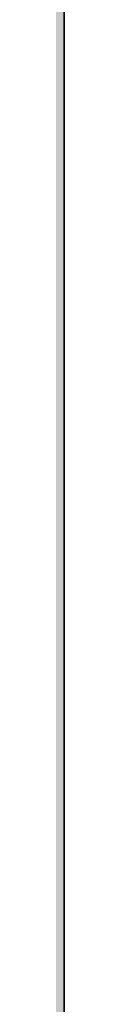
# Model space of a CAD drawing. Units: inches. Extents: x 2091 to 2899, y 967 to 2217.
# Tile 78 of 256: x 2212 to 2212, y 1114 to 1131. Entities that reach past the tile are written whole.
import ezdxf

# ---------------------------------------------------------------- set-up
doc = ezdxf.new("R2010")
doc.units = ezdxf.units.IN
doc.layers.add('A-WALL', color=7, linetype='Continuous', lineweight=35)
doc.layers.add('A-WALL-PATT', color=141, linetype='Continuous', lineweight=13, true_color=0xadddf7)

msp = doc.modelspace()

# ---------------------------------------------------------------- hatches: boundary and pattern name
at = {"layer": 'A-WALL-PATT'}
h = msp.add_hatch(color=256, dxfattribs=at)
h.dxf.hatch_style = 1
h.paths.add_polyline_path([(2212.144, 1941.419), (2387.644, 1941.419), (2387.644, 1824.419), (2392.144, 1824.419), (2392.144, 1941.419), (2609.644, 1941.419), (2609.644, 1825.919), (2614.144, 1825.919), (2614.144, 1941.419), (2794.144, 1941.419), (2794.144, 1928.762), (2803.144, 1928.762), (2803.144, 2050.919), (2203.144, 2050.919), (2203.144, 1900.758), (2212.144, 1900.758)])
h.paths.add_polyline_path([(2212.144, 1945.919), (2212.144, 2041.919), (2794.144, 2041.919), (2794.144, 1945.919), (2402.248, 1945.919), (2401.102, 1945.776), (2398.702, 1945.776)], flags=16)
h.paths.add_polyline_path([(2230.23, 1948.063), (2227.35, 1949.503), (2225.91, 1951.903), (2223.99, 1952.863), (2223.03, 1955.263), (2222.07, 1959.583), (2222.07, 1963.423), (2223.03, 1965.663), (2223.99, 1965.343), (2225.586, 1963.861), (2226.912, 1964.957), (2226.949, 1965.939), (2227.778, 1966.952), (2228.2, 1968.879), (2230.71, 1964.863), (2233.59, 1966.303), (2233.607, 1966.332), (2233.773, 1964.938), (2234.634, 1963.676), (2235.03, 1963.903), (2236.282, 1965.572), (2235.99, 1962.943), (2237.955, 1957.54), (2238.39, 1957.903), (2239.216, 1960.306), (2238.655, 1966.385), (2238.693, 1966.438), (2238.841, 1967.5), (2238.78, 1967.687), (2238.881, 1967.787), (2238.667, 1966.252), (2239.216, 1960.306), (2238.39, 1957.903), (2236.95, 1956.703), (2234.55, 1949.983)], flags=0)
h.paths.add_polyline_path([(2278.012, 1948.063), (2276.496, 1947.873), (2275.85, 1947.689), (2274.652, 1947.103)], flags=0)
h.paths.add_polyline_path([(2269.852, 1955.743), (2268.276, 1956.629), (2270.867, 1956.348), (2269.372, 1958.143), (2268.715, 1959.192), (2270.57, 1958.729), (2268.581, 1961.906), (2270.812, 1960.892), (2270.812, 1963.423), (2271.393, 1964.779), (2270.292, 1966.156), (2271.772, 1965.663), (2272.141, 1966.525), (2273.93, 1965.929), (2275.63, 1968.054), (2276.332, 1966.722), (2276.52, 1966.952), (2276.942, 1968.879), (2277.734, 1967.611), (2278.14, 1969.465), (2279.659, 1967.034), (2280.412, 1966.783), (2280.949, 1967.589), (2281.61, 1967.369), (2282.133, 1968.154), (2282.349, 1966.333), (2282.35, 1966.333), (2283.408, 1968.095), (2283.713, 1965.524), (2284.32, 1964.634), (2284.512, 1964.889), (2284.235, 1965.705), (2284.5, 1967.319), (2284.908, 1965.417), (2285.396, 1966.069), (2285.433, 1966.291), (2285.473, 1966.171), (2286.354, 1967.345), (2286.222, 1966.158), (2287.663, 1968.08), (2287.714, 1968.443), (2288.482, 1969.017), (2288.574, 1968.729), (2288.917, 1969.069), (2288.607, 1966.838), (2288.929, 1963.351), (2288.935, 1963.357), (2288.93, 1963.34), (2289.015, 1962.414), (2290.111, 1963.875), (2290.133, 1963.943), (2290.218, 1964.017), (2290.111, 1963.875), (2289.156, 1960.892), (2288.594, 1959.257), (2288.572, 1959.103), (2289.532, 1960.543), (2290.012, 1962.463), (2290.192, 1962.643), (2289.77, 1959.689), (2286.89, 1957.289), (2284.49, 1950.569), (2283.315, 1950.046), (2283.292, 1949.983), (2280.29, 1948.649), (2281.13, 1948.649), (2282.57, 1948.169), (2283.205, 1948.063), (2278.972, 1948.063), (2276.092, 1949.503), (2274.652, 1951.903), (2272.732, 1952.863)], flags=0)
h.paths.add_polyline_path([(2271.159, 1958.022), (2272.97, 1955.849), (2272.01, 1960.169), (2272.01, 1964.009), (2272.624, 1965.443), (2274.328, 1963.861), (2275.654, 1964.957), (2275.638, 1964.539), (2277.412, 1966.007), (2277.033, 1965.157), (2276.83, 1964.976), (2276.766, 1963.295), (2277.45, 1962.66), (2279.452, 1964.863), (2282.332, 1966.303), (2283.53, 1966.889), (2283.295, 1966.771), (2283.913, 1963.885), (2284.899, 1964.448), (2284.732, 1962.943), (2286.697, 1957.54), (2287.132, 1957.903), (2287.542, 1959.095), (2287.779, 1958.442), (2285.683, 1956.695), (2285.877, 1959.795), (2284.732, 1962.943), (2284.899, 1964.448), (2283.913, 1963.885), (2284.224, 1962.434), (2283.424, 1963.605), (2281.61, 1962.569), (2281.13, 1960.169), (2282.09, 1956.329), (2283.05, 1952.969), (2282.57, 1950.569), (2280.17, 1948.649), (2279.883, 1948.792), (2278.972, 1948.063), (2278.972, 1949.023), (2278.672, 1949.397), (2277.29, 1950.089), (2275.85, 1952.489), (2273.93, 1953.449), (2272.49, 1954.889), (2271.922, 1954.889), (2271.772, 1955.263)], flags=0)
h.paths.add_polyline_path([(2311.994, 1955.743), (2312.063, 1955.674), (2312.055, 1955.709)], flags=0)
h.paths.add_polyline_path([(2331.956, 1963.952), (2333.396, 1965.392), (2331.077, 1963.357), (2330.999, 1963.112)], flags=0)
h.paths.add_polyline_path([(2310.554, 1954.303), (2307.04, 1956.28), (2310.763, 1955.876), (2312.474, 1953.823), (2313.434, 1951.423), (2315.354, 1950.463), (2316.794, 1948.063), (2317.466, 1947.727), (2319.369, 1947.965), (2317.754, 1949.983), (2317.57, 1950.61), (2316.794, 1951.903), (2314.874, 1952.863), (2313.914, 1955.263), (2311.514, 1958.143), (2309.375, 1961.559), (2311.514, 1960.337), (2311.514, 1961.983), (2310.605, 1963.12), (2311.727, 1962.479), (2312.418, 1964.093), (2312.256, 1964.296), (2313.194, 1963.983), (2313.914, 1965.663), (2314.647, 1965.419), (2315.354, 1966.303), (2316.794, 1967.743), (2316.157, 1966.947), (2317.034, 1965.282), (2317.223, 1965.512), (2317.777, 1968.046), (2318.474, 1966.722), (2318.663, 1966.952), (2319.084, 1968.879), (2321.207, 1965.482), (2322.161, 1966.914), (2322.554, 1966.783), (2322.786, 1967.131), (2322.882, 1966.324), (2323.312, 1965.722), (2323.651, 1965.891), (2324.396, 1967.133), (2324.657, 1964.938), (2324.972, 1964.477), (2325.387, 1967.001), (2325.941, 1964.418), (2327.229, 1966.136), (2327.166, 1965.572), (2328.059, 1966.763), (2328.225, 1966.247), (2329.668, 1967.677), (2329.665, 1967.687), (2329.765, 1967.787), (2329.551, 1966.252), (2330.1, 1960.306), (2329.333, 1958.073), (2329.313, 1957.935), (2329.634, 1958.203), (2330.234, 1959.103), (2330.714, 1961.023), (2331.034, 1961.343), (2330.714, 1959.103), (2329.634, 1958.203), (2329.274, 1957.663), (2327.712, 1956.361), (2325.434, 1949.983), (2324.334, 1949.494), (2323.994, 1948.543), (2319.674, 1946.623), (2316.794, 1948.063), (2315.354, 1950.463), (2313.434, 1951.423)], flags=0)
h.paths.add_polyline_path([(2321.336, 1947.952), (2321.114, 1948.063), (2321.114, 1949.023), (2319.194, 1951.423), (2316.794, 1959.583), (2316.663, 1959.583), (2315.354, 1958.143), (2314.394, 1958.143), (2313.148, 1958.709), (2312.954, 1959.583), (2312.954, 1960.892), (2315.834, 1959.583), (2316.663, 1959.583), (2317.315, 1960.299), (2315.03, 1962.421), (2316.356, 1963.517), (2316.372, 1963.952), (2316.47, 1963.861), (2317.796, 1964.957), (2317.755, 1963.89), (2319.175, 1965.157), (2319.498, 1965.881), (2321.114, 1965.343), (2323.236, 1962.372), (2325.686, 1963.773), (2325.543, 1962.481), (2325.199, 1963.494), (2324.479, 1963.082), (2324.926, 1960.994), (2324.078, 1962.236), (2322.415, 1961.286), (2322.074, 1959.583), (2323.034, 1955.743), (2323.994, 1952.383), (2323.514, 1949.983), (2322.143, 1948.886), (2322.074, 1948.543)], flags=0)
h.paths.add_polyline_path([(2320.207, 1963.337), (2320.154, 1963.423), (2320.394, 1963.543)], flags=0)
h.paths.add_polyline_path([(2353.851, 1965.811), (2354.031, 1965.751), (2354.331, 1966.451), (2354.331, 1966.931)], flags=0)
h.paths.add_polyline_path([(2359.021, 1969.026), (2359.098, 1968.902), (2359.234, 1969.52), (2359.234, 1970)], flags=0)
h.paths.add_polyline_path([(2358.257, 1966.682), (2357.984, 1966.348), (2358.211, 1966.146), (2358.41, 1966.39)], flags=0)
h.paths.add_polyline_path([(2357.768, 1966.059), (2357.732, 1965.105), (2357.751, 1965.121), (2357.77, 1965.607), (2357.77, 1966.058)], flags=0)
h.paths.add_polyline_path([(2359.112, 1965.305), (2359.112, 1964.825), (2359.845, 1966.468), (2359.845, 1966.948)], flags=0)
h.paths.add_polyline_path([(2360.224, 1966.621), (2360.699, 1969.363), (2360.699, 1969.843), (2360.211, 1967.026), (2360.211, 1966.643)], flags=0)
h.paths.add_polyline_path([(2363.451, 1967.891), (2363.451, 1968.371), (2362.491, 1966.931), (2362.656, 1966.699)], flags=0)
h.paths.add_polyline_path([(2364.476, 1966.079), (2365.851, 1968.371), (2365.851, 1968.851), (2364.428, 1966.48)], flags=0)
h.paths.add_polyline_path([(2366.314, 1965.853), (2366.367, 1965.696), (2366.803, 1968.346), (2366.803, 1968.826)], flags=0)
h.paths.add_polyline_path([(2367.165, 1965.804), (2367.291, 1966.931), (2367.291, 1967.411), (2367.103, 1965.72)], flags=0)
h.paths.add_polyline_path([(2370.037, 1959.974), (2371.014, 1963.025), (2371.014, 1963.505), (2370.037, 1960.454)], flags=0)
h.paths.add_polyline_path([(2371.611, 1960.211), (2372.571, 1961.651), (2372.571, 1962.131), (2371.803, 1960.979)], flags=0)
h.paths.add_polyline_path([(2350.874, 1956.005), (2351.931, 1955.891), (2354.491, 1953.331), (2353.851, 1954.931), (2351.451, 1957.811), (2347.936, 1963.426), (2347.936, 1963.906), (2351.451, 1958.291), (2353.705, 1955.585), (2352.891, 1959.251), (2352.891, 1959.731), (2352.891, 1961.925), (2356.731, 1959.731), (2358.454, 1961.627), (2354.811, 1965.011), (2355.031, 1965.286), (2358.691, 1961.887), (2361.531, 1965.011), (2364.376, 1966.433), (2364.524, 1965.187), (2365.454, 1963.824), (2365.881, 1964.068), (2365.371, 1966.451), (2365.371, 1966.931), (2366.811, 1960.211), (2366.811, 1959.731), (2366.389, 1952.981), (2367.771, 1956.851), (2368.641, 1957.576), (2366.811, 1962.611), (2366.811, 1963.091), (2368.775, 1957.688), (2369.211, 1958.051), (2370.002, 1960.352), (2369.475, 1966.053), (2369.513, 1966.106), (2369.514, 1966.111), (2369.475, 1966.533), (2369.513, 1966.586), (2369.615, 1967.313), (2369.183, 1968.659), (2369.183, 1969.139), (2369.601, 1967.835), (2369.701, 1967.934), (2369.718, 1968.055), (2370.145, 1968.374), (2369.779, 1968.011), (2369.701, 1967.454), (2370.468, 1968.214), (2369.675, 1967.266), (2369.514, 1966.111), (2370.037, 1960.454), (2370.037, 1959.974), (2369.442, 1958.243), (2370.651, 1959.251), (2371.046, 1962.018), (2371.131, 1962.131), (2370.651, 1958.771), (2367.771, 1956.371), (2365.371, 1949.651), (2362.079, 1948.188), (2363.451, 1947.731), (2361.051, 1947.731), (2360.091, 1947.731), (2357.104, 1947.357), (2360.091, 1948.211), (2358.171, 1949.171), (2356.731, 1951.571), (2354.811, 1952.531), (2351.931, 1955.411)], flags=0)
h.paths.add_polyline_path([(2361.051, 1948.691), (2359.131, 1951.091), (2356.731, 1959.251), (2355.771, 1959.251), (2352.891, 1960.56), (2352.891, 1961.445), (2355.891, 1959.731), (2356.731, 1959.731), (2356.837, 1959.368), (2361.531, 1964.531), (2363.248, 1965.389), (2364.925, 1963.042), (2362.491, 1961.651), (2362.064, 1959.517), (2362.971, 1955.891), (2363.931, 1952.531), (2363.931, 1952.051), (2363.451, 1949.651), (2361.051, 1947.731)], flags=0)
h.paths.add_polyline_path([(2359.131, 1951.571), (2359.291, 1951.371), (2361.051, 1954.451), (2361.051, 1954.931)], flags=0)
h.paths.add_polyline_path([(2357.22, 1966.546), (2356.793, 1968.815), (2356.793, 1969.295), (2357.22, 1967.026)], flags=0)
h.paths.add_polyline_path([(2361.051, 1954.451), (2361.531, 1958.771), (2361.531, 1959.251), (2361.051, 1954.931)], flags=0)
h.paths.add_polyline_path([(2402.548, 1948.486), (2402.302, 1948.416), (2402.59, 1948.416)], flags=0)
h.paths.add_polyline_path([(2394.142, 1956.096), (2395.685, 1954.553), (2396.72, 1953.971), (2396.062, 1955.616), (2395.241, 1956.601), (2395.879, 1956.442), (2395.102, 1959.936), (2395.102, 1963.776), (2396.062, 1966.016), (2397.022, 1965.696), (2398.618, 1964.214), (2399.944, 1965.31), (2399.981, 1966.292), (2400.811, 1967.305), (2401.232, 1969.232), (2403.538, 1965.543), (2403.942, 1967.389), (2404.702, 1967.136), (2405.46, 1966.075), (2406.622, 1966.656), (2406.64, 1966.685), (2406.805, 1965.291), (2406.926, 1965.115), (2407.342, 1964.976), (2407.874, 1965.774), (2408.169, 1964.398), (2409.315, 1965.925), (2409.217, 1965.051), (2409.445, 1963.131), (2410.306, 1961.87), (2410.702, 1962.096), (2411.442, 1963.082), (2411.165, 1963.898), (2411.616, 1966.64), (2411.725, 1966.791), (2411.873, 1967.853), (2411.813, 1968.041), (2411.913, 1968.14), (2411.699, 1966.605), (2412.248, 1960.659), (2413.225, 1963.71), (2414.378, 1964.721), (2414.513, 1965.693), (2414.453, 1965.881), (2414.553, 1965.98), (2414.378, 1964.721), (2414.52, 1964.846), (2414.365, 1964.631), (2414.339, 1964.445), (2414.888, 1958.499), (2414.062, 1956.096), (2412.622, 1954.896), (2410.171, 1948.033), (2410.017, 1948.084), (2405.902, 1946.256), (2405.902, 1947.216), (2405.204, 1948.089), (2404.222, 1948.416), (2403.262, 1948.416), (2400.382, 1949.856), (2399.662, 1951.056), (2397.982, 1952.736), (2397.022, 1953.216), (2395.685, 1954.553), (2392.657, 1956.257)], flags=0)
h.paths.add_polyline_path([(2409.086, 1964.407), (2409.13, 1964.276), (2409.262, 1964.496)], flags=0)
h.paths.add_polyline_path([(2397.742, 1961.616), (2398.702, 1963.856), (2399.662, 1963.536), (2401.427, 1965.741), (2401.791, 1966.559), (2402.071, 1965.071), (2402.836, 1964.393), (2403.262, 1964.915), (2403.338, 1964.771), (2402.616, 1963.976), (2402.499, 1960.902), (2403.543, 1959.932), (2404.413, 1960.89), (2404.702, 1962.336), (2407.916, 1964.172), (2409.52, 1961.927), (2410.987, 1957.893), (2411.422, 1958.256), (2412.048, 1960.076), (2412.41, 1959.079), (2411.676, 1958.467), (2411.662, 1958.256), (2411.626, 1958.426), (2409.982, 1957.056), (2407.582, 1950.336), (2403.262, 1948.416), (2403.262, 1949.376), (2401.342, 1951.776), (2399.417, 1958.324), (2397.742, 1959.085), (2397.742, 1959.97), (2397.102, 1960.336), (2397.742, 1960.045)], flags=0)
h.paths.add_polyline_path([(2405.902, 1952.976), (2405.95, 1953.408), (2406.017, 1953.176)], flags=0)
h.paths.add_polyline_path([(2449.818, 1967.114), (2449.752, 1967.136), (2449.794, 1967.078)], flags=0)
h.paths.add_polyline_path([(2451.698, 1966.618), (2451.741, 1966.69), (2451.692, 1966.666)], flags=0)
h.paths.add_polyline_path([(2454.344, 1965.738), (2455.752, 1967.616), (2455.992, 1968.096), (2454.364, 1965.925)], flags=0)
h.paths.add_polyline_path([(2457.547, 1968.864), (2457.787, 1969.344), (2457.054, 1968.796), (2457.008, 1968.46)], flags=0)
h.paths.add_polyline_path([(2456.922, 1967.857), (2456.802, 1968.229), (2456.723, 1967.66)], flags=0)
h.paths.add_polyline_path([(2457.302, 1967.377), (2457.542, 1967.857), (2456.81, 1966.84), (2456.741, 1966.7), (2456.749, 1966.608)], flags=0)
h.paths.add_polyline_path([(2458.275, 1963.71), (2458.155, 1963.335), (2460.354, 1965.265), (2460.594, 1965.745)], flags=0)
h.paths.add_polyline_path([(2458.392, 1962.816), (2458.364, 1962.618), (2459.592, 1964.256), (2459.832, 1964.736)], flags=0)
h.paths.add_polyline_path([(2459.352, 1962.816), (2459.272, 1962.496), (2460.072, 1963.296), (2460.312, 1963.776)], flags=0)
h.paths.add_polyline_path([(2458.68, 1960.608), (2458.632, 1960.416), (2459.592, 1961.856), (2459.832, 1962.336)], flags=0)
h.paths.add_polyline_path([(2437.838, 1956.243), (2439.192, 1956.096), (2441.352, 1953.936), (2440.872, 1955.136), (2438.472, 1958.016), (2438.072, 1958.656), (2438.712, 1958.496), (2440.64, 1956.183), (2439.912, 1959.456), (2439.912, 1963.296), (2441.352, 1966.656), (2441.592, 1967.136), (2441.112, 1966.016), (2442.072, 1965.696), (2443.989, 1968.092), (2444.241, 1966.751), (2444.917, 1966.152), (2445.677, 1967.08), (2446.255, 1969.725), (2446.495, 1970.205), (2446.282, 1969.232), (2447.363, 1967.503), (2447.72, 1969.568), (2447.96, 1970.048), (2447.485, 1967.307), (2448.792, 1965.216), (2448.472, 1964.864), (2448.552, 1964.736), (2451.452, 1966.186), (2451.615, 1964.811), (2452.308, 1963.796), (2453.235, 1964.326), (2454.072, 1960.416), (2453.629, 1953.318), (2454.792, 1956.576), (2455.032, 1957.056), (2455.719, 1957.628), (2453.832, 1962.816), (2453.941, 1963.794), (2453.335, 1965.578), (2453.824, 1968.551), (2454.064, 1969.031), (2453.575, 1966.058), (2454.04, 1964.688), (2453.832, 1962.816), (2455.719, 1957.628), (2456.367, 1958.168), (2457.058, 1960.179), (2457.298, 1960.659), (2456.472, 1958.256), (2457.718, 1959.294), (2457.672, 1958.976), (2454.89, 1956.657), (2453.614, 1953.085), (2453.592, 1952.736), (2453.352, 1952.256), (2453.36, 1952.372), (2452.632, 1950.336), (2452.392, 1949.856), (2449.204, 1948.439), (2450.712, 1947.936), (2448.072, 1947.936), (2447.112, 1947.936), (2444.552, 1947.616), (2447.2, 1948.372), (2445.192, 1949.376), (2443.752, 1951.776), (2441.832, 1952.736), (2438.952, 1955.616)], flags=0)
h.paths.add_polyline_path([(2443.992, 1959.936), (2444.04, 1959.773), (2444.122, 1959.862)], flags=0)
h.paths.add_polyline_path([(2442.912, 1959.936), (2443.032, 1959.936), (2442.446, 1960.202)], flags=0)
h.paths.add_polyline_path([(2444.983, 1965.02), (2445.279, 1965.265), (2445.519, 1965.745), (2444.994, 1965.31)], flags=0)
h.paths.add_polyline_path([(2446.133, 1965.03), (2446.33, 1965.471), (2444.97, 1964.258), (2444.73, 1963.778)], flags=0)
h.paths.add_polyline_path([(2442.792, 1959.456), (2443.752, 1959.456), (2446.152, 1951.296), (2446.412, 1951.751), (2446.392, 1951.776), (2448.081, 1954.73), (2448.552, 1958.976), (2441.832, 1965.216), (2442.155, 1965.619), (2448.792, 1959.456), (2448.312, 1955.136), (2448.072, 1954.656), (2446.412, 1951.751), (2448.312, 1949.376), (2448.312, 1948.416), (2450.541, 1950.199), (2450.952, 1952.256), (2449.992, 1955.616), (2449.032, 1959.456), (2449.512, 1961.856), (2449.752, 1962.336), (2449.675, 1961.949), (2452.995, 1963.846), (2453.064, 1963.519), (2452.885, 1963.783), (2449.675, 1961.949), (2449.272, 1959.936), (2450.232, 1956.096), (2451.192, 1952.736), (2450.712, 1950.336), (2450.472, 1949.856), (2448.072, 1947.936), (2448.072, 1948.536), (2445.432, 1949.856), (2443.992, 1952.256), (2442.072, 1953.216), (2441.112, 1955.616), (2440.152, 1959.936), (2440.152, 1960.656)], flags=0)
h.paths.add_polyline_path([(2456.692, 1966.986), (2457.608, 1968.081), (2457.848, 1968.561), (2456.932, 1967.466)], flags=0)
h.paths.add_polyline_path([(2489.897, 1966.58), (2489.943, 1966.189), (2490.747, 1967.53), (2491.319, 1968.951)], flags=0)
h.paths.add_polyline_path([(2473.562, 1956.407), (2477.14, 1956.019), (2476.955, 1956.241), (2475.108, 1957.28), (2476.347, 1956.97), (2475.187, 1958.824), (2476.919, 1958.391), (2475.412, 1960.799), (2477.787, 1959.719), (2477.787, 1962.25), (2477.637, 1962.438), (2477.823, 1962.332), (2478.359, 1963.584), (2478.359, 1963.671), (2477.324, 1964.965), (2478.715, 1964.501), (2479.319, 1965.911), (2480.279, 1965.591), (2481.784, 1967.472), (2482.116, 1965.705), (2482.881, 1965.028), (2483.209, 1965.429), (2483.22, 1965.715), (2483.076, 1965.989), (2483.712, 1966.766), (2484.13, 1968.679), (2484.702, 1970.1), (2484.489, 1969.127), (2486.503, 1965.905), (2487.387, 1965.61), (2488.153, 1966.759), (2488.717, 1965.97), (2489.2, 1966.212), (2489.331, 1965.111), (2490.394, 1963.622), (2490.661, 1963.775), (2490.494, 1964.554), (2490.923, 1963.925), (2491.319, 1964.151), (2491.333, 1964.17), (2491.21, 1964.532), (2491.282, 1964.966), (2491.426, 1964.293), (2494.076, 1967.828), (2494.498, 1966.515), (2494.598, 1966.614), (2494.689, 1967.27), (2495.107, 1967.582), (2495.13, 1967.748), (2495.07, 1967.936), (2495.17, 1968.035), (2495.032, 1967.044), (2495.754, 1967.759), (2494.982, 1966.686), (2494.956, 1966.5), (2495.479, 1960.837), (2495.91, 1962.184), (2496.482, 1963.605), (2496.073, 1962.327), (2496.769, 1962.938), (2496.599, 1962.711), (2496.119, 1959.351), (2496.733, 1960.272), (2496.987, 1961.29), (2497.559, 1962.711), (2497.079, 1960.791), (2496.507, 1959.37), (2495.547, 1957.93), (2492.759, 1955.606), (2490.839, 1950.231), (2490.267, 1948.81), (2485.947, 1946.89), (2483.067, 1948.33), (2481.627, 1950.73), (2479.707, 1951.69), (2476.827, 1954.57)], flags=0)
h.paths.add_polyline_path([(2485.577, 1948.313), (2485.559, 1948.311), (2485.579, 1948.311)], flags=0)
h.paths.add_polyline_path([(2478.645, 1954.551), (2478.109, 1956.963), (2479.319, 1955.511), (2480.279, 1953.111), (2482.199, 1952.151), (2483.639, 1949.751), (2486.519, 1948.311), (2486.519, 1949.271), (2484.739, 1951.496), (2484.027, 1950.25), (2481.627, 1958.41), (2482.375, 1959.233), (2482.199, 1959.831), (2483.198, 1960.929), (2479.707, 1964.17), (2480.603, 1965.29), (2481.875, 1964.109), (2482.666, 1964.764), (2482.615, 1963.422), (2482.989, 1963.075), (2484.008, 1963.984), (2484.684, 1965.498), (2484.58, 1965.405), (2485.357, 1967.147), (2485.121, 1965.781), (2486.427, 1963.69), (2488.145, 1964.549), (2489.822, 1962.202), (2490.747, 1962.73), (2492, 1964.4), (2492.076, 1965.087), (2492.213, 1964.684), (2492.485, 1965.047), (2492.279, 1963.191), (2494.244, 1957.788), (2494.563, 1958.054), (2494.933, 1959.133), (2495.505, 1960.554), (2494.679, 1958.151), (2494.107, 1956.73), (2494.563, 1958.054), (2493.409, 1957.092), (2491.707, 1961.77), (2492, 1964.4), (2490.747, 1962.73), (2487.712, 1960.996), (2487.479, 1959.831), (2488.439, 1955.991), (2489.399, 1952.631), (2488.919, 1950.231), (2488.577, 1949.957), (2488.347, 1948.81), (2487.652, 1948.254), (2487.479, 1948.311), (2486.519, 1948.311), (2483.639, 1949.751), (2482.199, 1952.151), (2480.279, 1953.111), (2478.839, 1954.551)], flags=0)
h.paths.add_polyline_path([(2526.648, 1966.988), (2526.517, 1967.031), (2526.6, 1966.915)], flags=0)
h.paths.add_polyline_path([(2528.471, 1966.447), (2528.574, 1966.62), (2528.457, 1966.561)], flags=0)
h.paths.add_polyline_path([(2534.133, 1967.496), (2534.157, 1967.543), (2534.06, 1967.408)], flags=0)
h.paths.add_polyline_path([(2536.162, 1964.051), (2535.157, 1962.711), (2535.101, 1962.316), (2536.117, 1963.671), (2536.421, 1964.278)], flags=0)
h.paths.add_polyline_path([(2535.157, 1959.831), (2536.117, 1961.271), (2536.597, 1962.231), (2535.253, 1960.215)], flags=0)
h.paths.add_polyline_path([(2513.249, 1956.285), (2516.221, 1955.963), (2514.997, 1957.431), (2514.196, 1958.712), (2515.477, 1958.391), (2516.932, 1956.646), (2516.437, 1958.871), (2516.437, 1962.711), (2516.873, 1963.727), (2515.346, 1965.635), (2517.397, 1964.951), (2517.877, 1966.071), (2518.357, 1967.031), (2517.877, 1965.911), (2518.837, 1965.591), (2520.487, 1967.653), (2520.766, 1966.166), (2521.53, 1965.489), (2521.781, 1965.795), (2521.801, 1966.307), (2521.478, 1966.921), (2521.246, 1967.126), (2521.178, 1967.491), (2521.478, 1966.921), (2522.01, 1966.449), (2522.257, 1966.75), (2522.78, 1969.14), (2523.26, 1970.1), (2523.047, 1969.127), (2524.673, 1966.526), (2526.037, 1966.071), (2526.795, 1965.01), (2527.977, 1965.601), (2528.14, 1964.227), (2528.665, 1963.458), (2529.389, 1963.872), (2529.33, 1964.147), (2529.481, 1963.925), (2529.877, 1964.151), (2529.984, 1964.293), (2529.789, 1965.203), (2530.062, 1964.398), (2532.802, 1968.051), (2533.148, 1966.976), (2533.248, 1967.075), (2533.339, 1967.731), (2533.673, 1967.98), (2533.728, 1968.035), (2533.514, 1966.5), (2534.025, 1960.972), (2534.56, 1962.645), (2535.04, 1963.605), (2534.063, 1960.554), (2533.237, 1958.151), (2534.288, 1959.027), (2534.197, 1958.391), (2531.513, 1956.154), (2529.397, 1950.231), (2528.917, 1949.271), (2526.449, 1948.174), (2527.477, 1947.831), (2530.357, 1947.351), (2524.597, 1947.351), (2521.717, 1948.791), (2520.277, 1951.191), (2518.357, 1952.151), (2515.477, 1955.031)], flags=0)
h.paths.add_polyline_path([(2523.935, 1967.19), (2523.62, 1966.484), (2523.77, 1966.242)], flags=0)
h.paths.add_polyline_path([(2518.837, 1953.111), (2517.877, 1955.511), (2516.885, 1959.977), (2516.917, 1959.962), (2516.917, 1962.025), (2520.757, 1959.831), (2522.025, 1961.226), (2518.357, 1964.631), (2519.003, 1965.438), (2520.433, 1964.109), (2521.301, 1964.827), (2521.245, 1963.355), (2525.638, 1959.276), (2526.037, 1961.271), (2529.397, 1963.191), (2530.65, 1964.861), (2530.665, 1964.998), (2530.692, 1964.917), (2531.088, 1965.445), (2530.946, 1964.169), (2530.692, 1964.917), (2529.397, 1963.191), (2526.363, 1961.457), (2526.037, 1959.831), (2526.997, 1955.991), (2527.957, 1952.631), (2527.477, 1950.231), (2527.134, 1949.957), (2526.974, 1949.154), (2526.697, 1949.031), (2524.597, 1947.351), (2524.597, 1948.311), (2524.277, 1948.711), (2522.197, 1949.751), (2520.757, 1952.151)], flags=0)
h.paths.add_polyline_path([(2520.277, 1958.871), (2520.853, 1959.505), (2523.157, 1951.671), (2524.614, 1954.22), (2524.597, 1954.071), (2522.677, 1950.711)], flags=0)
h.paths.add_polyline_path([(2559.371, 1966.311), (2559.398, 1966.325), (2559.402, 1966.345)], flags=0)
h.paths.add_polyline_path([(2549.771, 1957.191), (2552.651, 1954.311), (2552.134, 1955.603), (2550.611, 1957.431), (2547.096, 1963.046), (2545.776, 1965.206), (2549.291, 1959.591), (2551.691, 1956.711), (2550.793, 1960.752), (2550.731, 1960.78), (2550.731, 1964.871), (2551.691, 1967.111), (2552.651, 1966.791), (2554.247, 1965.309), (2555.034, 1965.96), (2555.582, 1966.645), (2555.61, 1967.387), (2556.439, 1968.401), (2556.861, 1970.327), (2559.371, 1966.311), (2560.691, 1964.151), (2562.409, 1965.01), (2561.651, 1966.071), (2560.331, 1968.231), (2561.758, 1966.233), (2562.347, 1967.116), (2562.434, 1966.387), (2563.128, 1965.37), (2563.571, 1965.591), (2563.588, 1965.62), (2563.363, 1967.524), (2563.722, 1965.844), (2565.06, 1968.073), (2564.733, 1965.129), (2565.118, 1963.333), (2567.445, 1966.436), (2567.316, 1967.833), (2567.354, 1967.886), (2567.502, 1968.948), (2567.441, 1969.136), (2567.542, 1969.235), (2567.328, 1967.7), (2567.877, 1961.754), (2568.747, 1964.47), (2568.636, 1965.673), (2568.674, 1965.726), (2568.822, 1966.788), (2568.761, 1966.976), (2568.862, 1967.075), (2568.648, 1965.54), (2568.726, 1964.693), (2568.854, 1964.805), (2568.747, 1964.47), (2568.817, 1963.706), (2568.971, 1963.911), (2568.866, 1963.177), (2569.197, 1959.594), (2568.371, 1957.191), (2566.931, 1955.991), (2564.62, 1949.521), (2564.651, 1949.511), (2564.617, 1949.511), (2564.531, 1949.271), (2560.211, 1947.351), (2557.331, 1948.791), (2556.045, 1950.934), (2556.011, 1950.951), (2555.857, 1951.208), (2553.971, 1952.151), (2551.091, 1955.031), (2546.65, 1957.53)], flags=0)
h.paths.add_polyline_path([(2567.026, 1959.33), (2567.035, 1959.305), (2567.051, 1959.351)], flags=0)
h.paths.add_polyline_path([(2551.968, 1962.518), (2553.011, 1964.951), (2553.971, 1964.631), (2555.567, 1963.149), (2556.893, 1964.246), (2556.93, 1965.227), (2557.144, 1965.489), (2556.42, 1966.131), (2556.391, 1966.105), (2556.38, 1966.166), (2556.42, 1966.131), (2556.952, 1966.605), (2557.092, 1966.919), (2557.571, 1966.01), (2557.759, 1966.241), (2557.418, 1964.68), (2556.893, 1964.246), (2556.807, 1961.998), (2560.691, 1958.391), (2560.636, 1957.893), (2560.811, 1957.191), (2561.771, 1953.831), (2561.291, 1951.431), (2559.11, 1949.687), (2559.156, 1949.629), (2563.027, 1951.349), (2562.611, 1949.271), (2560.211, 1947.351), (2560.211, 1948.311), (2559.251, 1949.511), (2558.891, 1949.511), (2558.891, 1949.961), (2558.291, 1950.711), (2558.054, 1951.518), (2556.971, 1952.871), (2555.068, 1959.341), (2552.051, 1961.065), (2552.051, 1962.471)], flags=0)
h.paths.add_polyline_path([(2588.33, 1958.391), (2588.61, 1958.111), (2588.553, 1958.367)], flags=0)
h.paths.add_polyline_path([(2594.745, 1950.493), (2593.958, 1953.172), (2593.13, 1954.551), (2591.21, 1955.511), (2590.25, 1957.911), (2588.309, 1960.24), (2586.177, 1961.209), (2587.85, 1960.791), (2587.253, 1961.744), (2588.441, 1961.065), (2588.441, 1962.656), (2588.422, 1962.665), (2588.441, 1962.711), (2586.914, 1964.62), (2588.877, 1963.728), (2589.29, 1964.692), (2589.29, 1966.071), (2590.25, 1968.311), (2591.21, 1967.991), (2592.806, 1966.509), (2594.132, 1967.606), (2594.169, 1968.587), (2594.999, 1969.601), (2595.42, 1971.527), (2597.93, 1967.511), (2600.81, 1968.951), (2600.827, 1968.98), (2600.993, 1967.587), (2601.854, 1966.325), (2602.107, 1966.47), (2602.236, 1967.255), (2602.357, 1966.693), (2603.502, 1968.221), (2603.21, 1965.591), (2605.175, 1960.188), (2605.507, 1960.465), (2605.026, 1965.673), (2605.064, 1965.726), (2605.212, 1966.788), (2605.152, 1966.976), (2605.252, 1967.075), (2605.343, 1967.731), (2605.953, 1968.187), (2605.875, 1969.033), (2605.913, 1969.086), (2606.061, 1970.148), (2606, 1970.336), (2606.101, 1970.435), (2605.887, 1968.9), (2606.436, 1962.954), (2605.61, 1960.551), (2605.997, 1960.874), (2606.564, 1962.645), (2608.241, 1964.117), (2608.01, 1963.191), (2607.05, 1961.751), (2606.631, 1961.402), (2606.201, 1958.391), (2603.321, 1955.991), (2600.921, 1949.271), (2596.601, 1947.351), (2593.721, 1948.791), (2592.857, 1950.231), (2592.65, 1950.231)], flags=0)
h.paths.add_polyline_path([(2596.601, 1947.351), (2596.601, 1948.311), (2594.681, 1950.711), (2596.155, 1953.29), (2595.53, 1954.071), (2593.199, 1961.996), (2592.651, 1962.505), (2591.78, 1963.003), (2593.283, 1964.246), (2593.32, 1965.227), (2594.15, 1966.241), (2594.571, 1968.167), (2596.183, 1965.589), (2596.951, 1966.435), (2598.041, 1966.071), (2598.799, 1965.01), (2599.961, 1965.591), (2599.979, 1965.62), (2600.144, 1964.227), (2601.005, 1962.965), (2601.401, 1963.191), (2602.653, 1964.861), (2602.361, 1962.231), (2603.793, 1958.295), (2601.978, 1953.212), (2601.946, 1952.709), (2599.469, 1951.608), (2599.001, 1949.271)], flags=0)
h.paths.add_polyline_path([(2597.561, 1958.871), (2597.671, 1959.419), (2597.595, 1958.736)], flags=0)
h.paths.add_polyline_path([(2623.666, 1961.254), (2625.519, 1960.791), (2624.966, 1961.676), (2627.199, 1960.66), (2627.199, 1961.151), (2626.959, 1962.231), (2626.959, 1963.491), (2625.582, 1965.212), (2626.959, 1964.425), (2626.959, 1965.831), (2626.869, 1965.861), (2627.919, 1968.311), (2628.879, 1967.991), (2630.475, 1966.509), (2631.801, 1967.606), (2631.838, 1968.587), (2632.668, 1969.601), (2633.089, 1971.527), (2635.599, 1967.511), (2638.479, 1968.951), (2638.497, 1968.98), (2638.662, 1967.587), (2639.176, 1966.833), (2639.78, 1967.84), (2640.026, 1966.693), (2641.171, 1968.221), (2640.879, 1965.591), (2641.114, 1964.945), (2641.411, 1965.341), (2641.308, 1964.412), (2642.844, 1960.188), (2643.279, 1960.551), (2644.085, 1962.895), (2643.784, 1966.153), (2643.807, 1966.185), (2643.601, 1968.418), (2643.523, 1968.661), (2643.73, 1970.148), (2643.67, 1970.336), (2643.77, 1970.435), (2643.556, 1968.9), (2643.601, 1968.418), (2643.91, 1967.456), (2644.01, 1967.555), (2643.812, 1966.132), (2644.105, 1962.954), (2644.239, 1961.351), (2644.719, 1961.751), (2645.033, 1962.222), (2645.322, 1963.125), (2646.076, 1963.787), (2645.033, 1962.222), (2644.345, 1960.074), (2643.519, 1957.671), (2642.079, 1956.471), (2639.72, 1949.864), (2639.876, 1949.838), (2635.359, 1947.831), (2632.479, 1949.271), (2631.039, 1951.671), (2629.119, 1952.631), (2628.159, 1955.031), (2625.759, 1957.911)], flags=0)
h.paths.add_polyline_path([(2627.816, 1956.574), (2627.374, 1958.566), (2626.376, 1959.763), (2627.199, 1959.351), (2627.374, 1958.566), (2627.919, 1957.911), (2628.879, 1955.511), (2630.799, 1954.551), (2632.239, 1952.151), (2633.315, 1951.613), (2631.039, 1959.351), (2631.498, 1959.856), (2630.799, 1962.231), (2631.45, 1962.947), (2630.715, 1963.629), (2632.041, 1964.726), (2632.078, 1965.707), (2632.292, 1965.969), (2631.705, 1966.489), (2633.136, 1967.766), (2633.329, 1968.647), (2634.675, 1966.494), (2635.208, 1967.081), (2636.799, 1966.551), (2637.676, 1967.867), (2638.994, 1966.022), (2639.705, 1966.429), (2641.119, 1959.831), (2640.93, 1956.806), (2639.439, 1952.631), (2638.227, 1952.093), (2637.759, 1949.751), (2635.359, 1947.831), (2635.359, 1948.791), (2633.439, 1951.191), (2633.315, 1951.613), (2632.239, 1952.151), (2630.799, 1954.551), (2628.879, 1955.511)], flags=0)
h.paths.add_polyline_path([(2637.759, 1953.831), (2637.279, 1955.511), (2636.319, 1959.351), (2636.799, 1961.751), (2639.234, 1963.142), (2637.557, 1965.49), (2638.739, 1966.081), (2638.902, 1964.707), (2639.763, 1963.445), (2636.799, 1961.751), (2636.532, 1960.418), (2637.039, 1958.391), (2637.999, 1955.031)], flags=0)
h.paths.add_polyline_path([(2668.567, 1951.431), (2667.607, 1953.831), (2665.207, 1956.711), (2662.294, 1961.365), (2665.447, 1959.591), (2666.647, 1958.391), (2666.647, 1959.975), (2666.058, 1960.682), (2666.647, 1960.345), (2666.647, 1961.991), (2666.7, 1962.114), (2666.407, 1963.431), (2666.407, 1967.271), (2667.367, 1969.511), (2668.327, 1969.191), (2669.923, 1967.709), (2671.249, 1968.806), (2671.286, 1969.787), (2672.116, 1970.801), (2672.537, 1972.727), (2675.047, 1968.711), (2677.927, 1970.151), (2677.945, 1970.18), (2678.11, 1968.787), (2678.971, 1967.525), (2679.367, 1967.751), (2680.62, 1969.421), (2680.327, 1966.791), (2682.292, 1961.388), (2682.727, 1961.751), (2683.358, 1963.587), (2683.232, 1964.953), (2683.27, 1965.006), (2683.393, 1965.889), (2683.36, 1966.249), (2683.358, 1966.256), (2683.359, 1966.257), (2682.992, 1970.233), (2683.03, 1970.286), (2683.178, 1971.348), (2683.118, 1971.536), (2683.218, 1971.635), (2683.004, 1970.1), (2683.359, 1966.257), (2683.458, 1966.355), (2683.393, 1965.889), (2683.414, 1965.665), (2684.424, 1966.872), (2683.553, 1964.154), (2683.358, 1963.587), (2683.793, 1958.874), (2682.967, 1956.471), (2681.527, 1955.271), (2680.109, 1951.3), (2680.085, 1950.912), (2679.977, 1950.93), (2679.127, 1948.551), (2674.807, 1946.631), (2671.927, 1948.071), (2670.487, 1950.471)], flags=0)
h.paths.add_polyline_path([(2671.936, 1953.227), (2671.687, 1953.351), (2670.247, 1955.751), (2668.327, 1956.711), (2667.357, 1959.138), (2669.527, 1958.151), (2670.487, 1958.151), (2671.479, 1959.242), (2670.684, 1961.945), (2668.89, 1963.612), (2667.307, 1964.331), (2668.567, 1963.911), (2668.831, 1964.241), (2670.247, 1963.431), (2672.422, 1965.823), (2672.777, 1967.447), (2673.234, 1966.716), (2674.412, 1968.012), (2673.981, 1965.522), (2675.287, 1963.431), (2675.554, 1963.564), (2675.932, 1965.456), (2676.247, 1965.351), (2677.005, 1964.29), (2678.167, 1964.871), (2679.607, 1967.271), (2680.327, 1963.911), (2680.307, 1963.577), (2680.347, 1963.458), (2680.86, 1964.141), (2680.567, 1961.511), (2681.104, 1960.037), (2678.887, 1953.831), (2677.092, 1953.033), (2677.687, 1950.951), (2677.207, 1948.551), (2674.807, 1946.631), (2674.807, 1947.591), (2672.887, 1949.991)], flags=0)
h.paths.add_polyline_path([(2673.985, 1951.911), (2674.567, 1952.931), (2674.567, 1951.911), (2676.967, 1953.831), (2677.447, 1956.231), (2676.487, 1959.591), (2676.247, 1960.551), (2679.73, 1962.541), (2680.059, 1961.002), (2679.211, 1962.245), (2676.247, 1960.551), (2676.487, 1959.591), (2677.447, 1956.231), (2676.967, 1953.831), (2674.567, 1951.911)], flags=0)
h.paths.add_polyline_path([(2707.479, 1952.815), (2706.519, 1955.215), (2705.559, 1959.535), (2705.559, 1963.375), (2706.519, 1965.615), (2707.479, 1965.295), (2709.075, 1963.813), (2710.401, 1964.909), (2710.438, 1965.891), (2711.268, 1966.904), (2711.689, 1968.831), (2714.199, 1964.815), (2717.079, 1966.255), (2717.097, 1966.284), (2717.262, 1964.89), (2718.123, 1963.628), (2718.519, 1963.855), (2719.771, 1965.524), (2719.479, 1962.895), (2721.444, 1957.492), (2721.879, 1957.855), (2722.705, 1960.258), (2722.144, 1966.337), (2722.182, 1966.39), (2722.33, 1967.452), (2722.27, 1967.639), (2722.37, 1967.739), (2722.156, 1966.204), (2722.705, 1960.258), (2721.879, 1957.855), (2720.439, 1956.655), (2718.039, 1949.935), (2713.719, 1948.015), (2710.839, 1949.455), (2709.399, 1951.855)], flags=0)
h.paths.add_polyline_path([(2749.301, 1952.815), (2748.341, 1955.215), (2747.381, 1959.535), (2747.381, 1963.375), (2748.341, 1965.615), (2749.301, 1965.295), (2750.897, 1963.813), (2752.223, 1964.909), (2752.26, 1965.891), (2753.09, 1966.904), (2753.511, 1968.831), (2756.021, 1964.815), (2758.901, 1966.255), (2758.919, 1966.284), (2759.084, 1964.89), (2759.945, 1963.628), (2760.341, 1963.855), (2761.593, 1965.524), (2761.301, 1962.895), (2763.266, 1957.492), (2763.701, 1957.855), (2764.527, 1960.258), (2763.966, 1966.337), (2764.004, 1966.39), (2764.152, 1967.452), (2764.092, 1967.639), (2764.192, 1967.739), (2763.978, 1966.204), (2764.527, 1960.258), (2763.701, 1957.855), (2762.261, 1956.655), (2759.861, 1949.935), (2755.541, 1948.015), (2752.661, 1949.455), (2751.221, 1951.855)], flags=0)
h.paths.add_polyline_path([(2212.144, 1819.935), (2203.144, 1819.935), (2203.144, 1739.98), (2212.144, 1739.98), (2212.144, 1780.919), (2392.144, 1780.919), (2392.144, 1783.919), (2212.144, 1783.919)])
h.paths.add_polyline_path([(2803.144, 1847.939), (2794.144, 1847.939), (2794.144, 1785.419), (2609.644, 1785.419), (2493.876, 1785.419), (2493.876, 1780.919), (2609.644, 1780.919), (2794.144, 1780.919), (2794.144, 1696.919), (2609.376, 1696.919), (2609.376, 1742.919), (2604.876, 1742.919), (2604.876, 1644.419), (2609.376, 1644.419), (2609.376, 1692.419), (2794.144, 1692.419), (2794.144, 1668.165), (2803.144, 1668.165)])
h.paths.add_polyline_path([(2392.144, 1740.419), (2387.644, 1740.419), (2387.644, 1629.419), (2212.144, 1629.419), (2212.144, 1659.156), (2203.144, 1659.156), (2203.144, 1494.089), (2212.144, 1494.089), (2212.144, 1627.919), (2392.144, 1627.919)])
h.paths.add_polyline_path([(2457.876, 1780.919), (2453.376, 1780.919), (2453.376, 1644.419), (2568.876, 1644.419), (2568.876, 1648.919), (2457.876, 1648.919)])
h.paths.add_polyline_path([(2545.144, 1591.919), (2540.644, 1591.919), (2540.644, 1567.919), (2468.644, 1567.919), (2468.644, 1627.919), (2509.144, 1627.919), (2509.144, 1632.419), (2464.144, 1632.419), (2464.144, 1563.419), (2545.144, 1563.419)])
h.paths.add_polyline_path([(2268.644, 1555.919), (2212.144, 1555.919), (2212.144, 1551.419), (2268.644, 1551.419)], flags=17)
h.paths.add_polyline_path([(2212.144, 1413.266), (2203.144, 1413.266), (2203.144, 1233.07), (2212.144, 1233.07)])
h.paths.add_polyline_path([(2267.644, 1351.919), (2212.144, 1351.919), (2212.144, 1347.419), (2267.644, 1347.419)], flags=17)
h.paths.add_polyline_path([(2456.644, 1489.419), (2452.144, 1489.419), (2452.144, 1351.919), (2312.644, 1351.919), (2312.644, 1347.419), (2456.644, 1347.419)])
h.paths.add_polyline_path([(2472.37, 1455.419), (2467.87, 1455.419), (2467.87, 1347.419), (2472.37, 1347.419)])
h.paths.add_polyline_path([(2794.144, 1351.919), (2543.37, 1351.919), (2543.37, 1347.419), (2794.144, 1347.419)], flags=17)
h.paths.add_polyline_path([(2312.644, 1347.419), (2308.144, 1347.419), (2308.144, 1302.162), (2308.342, 1302.164), (2308.144, 1298.169), (2308.144, 1275.419), (2212.144, 1275.419), (2212.144, 1270.919), (2312.644, 1270.919)], flags=17)
h.paths.add_polyline_path([(2212.144, 1152.247), (2203.144, 1152.247), (2203.144, 1090.919), (2803.144, 1090.919), (2803.144, 1392.714), (2794.144, 1392.714), (2794.144, 1143.419), (2548.032, 1143.419), (2548.032, 1138.919), (2794.144, 1138.919), (2794.144, 1099.919), (2212.144, 1099.919)])
h.paths.add_polyline_path([(2471.532, 1266.329, 0.031658), (2467.032, 1269.946), (2467.032, 1143.419), (2471.532, 1143.419), (2471.532, 1148.819)], flags=17)
h.paths.add_polyline_path([(2803.144, 1587.341), (2794.144, 1587.341), (2794.144, 1473.537), (2803.144, 1473.537)])
h.paths.add_polyline_path([(2794.144, 1536.419), (2651.144, 1536.419), (2651.144, 1531.919), (2794.144, 1531.919)])
h.paths.add_polyline_path([(2614.144, 1620.419), (2609.644, 1620.419), (2609.644, 1536.419), (2614.144, 1536.419)])
h.paths.add_polyline_path([(2271.083, 1964.317), (2776.853, 1964.317), (2776.853, 2037.17), (2271.083, 2037.17)], flags=8)
h.paths.add_polyline_path([(2380.649, 1536.824), (2461.041, 1536.824), (2461.041, 1554.653), (2380.649, 1554.653)], flags=9)
h.paths.add_polyline_path([(2203.655, 1608.815), (2316.118, 1608.815), (2316.118, 1621.918), (2203.655, 1621.918)], flags=24)
h.paths.add_polyline_path([(2212.677, 1313.504), (2282.592, 1313.504), (2282.592, 1322.745), (2212.677, 1322.745)], flags=24)
h.paths.add_polyline_path([(2457.112, 1114.779), (2558.482, 1114.779), (2558.482, 1142.22), (2457.112, 1142.22)], flags=25)
h.paths.add_polyline_path([(2473.442, 1273.01), (2604.641, 1273.01), (2604.641, 1318.347), (2473.442, 1318.347)], flags=25)
h.paths.add_polyline_path([(2638.876, 1626.977), (2684.25, 1627.977), (2684.038, 1637.597), (2638.664, 1636.598)], flags=9)
h.paths.add_polyline_path([(2537.591, 1453.793), (2628.39, 1453.793), (2628.39, 1475.345), (2537.591, 1475.345)], flags=9)
h.paths.add_polyline_path([(2504.138, 1714.632), (2554.647, 1714.632), (2554.647, 1730.238), (2504.138, 1730.238)], flags=25)
h.paths.add_polyline_path([(2487.501, 1575.652), (2535.097, 1575.652), (2535.097, 1598.378), (2487.501, 1598.378)], flags=25)
h.paths.add_polyline_path([(2709.099, 1735.71), (2740.017, 1735.71), (2740.017, 1749.938), (2709.099, 1749.938)], flags=25)
h.paths.add_polyline_path([(2442.438, 1792.172), (2564.729, 1792.172), (2564.729, 1842), (2442.438, 1842)], flags=9)
h.paths.add_polyline_path([(2655.816, 1809.644), (2789.52, 1806.694), (2790.085, 1832.292), (2656.381, 1835.242)], flags=25)
h.paths.add_polyline_path([(2234.843, 1797.72), (2368.593, 1794.769), (2369.161, 1820.504), (2235.411, 1823.455)], flags=9)
h.paths.add_polyline_path([(2245.138, 1644.006), (2398.428, 1640.624), (2398.995, 1666.325), (2245.706, 1669.707)], flags=9)
h.paths.add_polyline_path([(2306.143, 1431.169), (2413.768, 1428.794), (2414.333, 1454.392), (2306.708, 1456.766)], flags=9)
h.paths.add_polyline_path([(2306.835, 1458.233), (2393.38, 1456.323), (2393.933, 1481.354), (2307.387, 1483.264)], flags=9)

# ---------------------------------------------------------------- linework, layer by layer
at = {"layer": 'A-WALL'}
msp.add_line((2212.144, 1099.919), (2212.144, 1627.919), dxfattribs=at)

doc.saveas('drawing.dxf')
